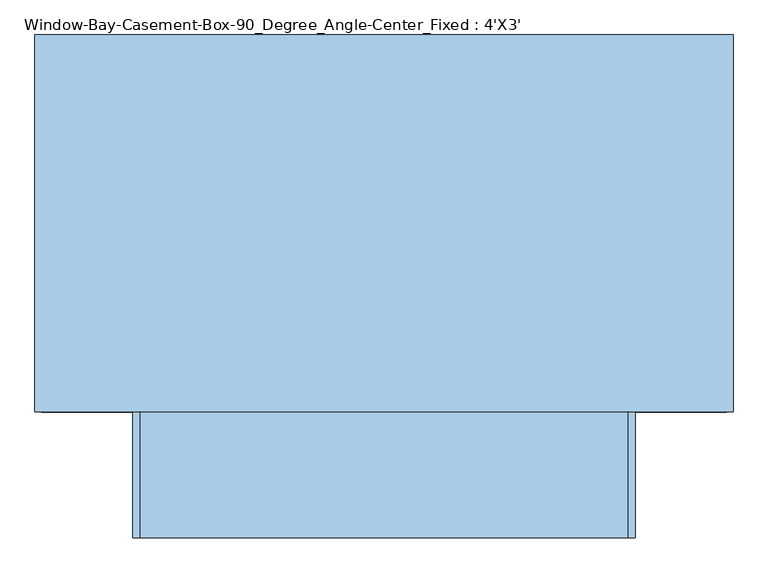
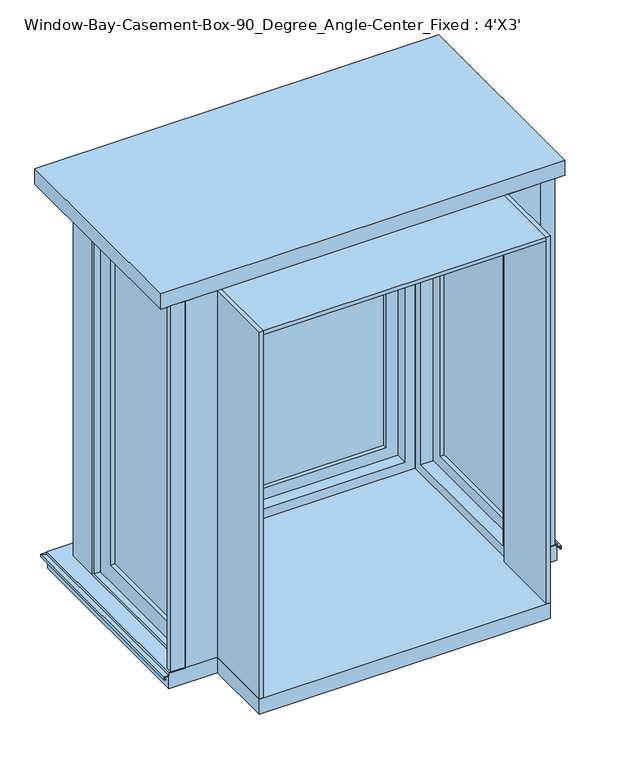
"""IFC4 building model written with IfcOpenShell, lengths in millimetres: window geometry, Window-Bay-Casement-Box-90_Degree_Angle-Center_Fixed : 4'X3'."""

from ifc_helpers import new_model, si_unit, frame, origin, place, context, project, spatial, polyline, outline, extrude, faceted_brep, source, transform, mapped, element, save


def window_bay_casement_box_90_degree_angle_center_fixed_4_x3_2dea7aab(model_context):
    return source(origin(), model_context, "Body", "SolidModel", [
        extrude(outline(polyline([(-558.8, 114.3), (-603.25, 114.3), (-603.25, 133.35), (-558.8, 133.35), (-558.8, 114.3)])), frame((0.0, 0.0, 663.1486341), z_axis=(0.0, 0.0, 1.0), x_axis=(1.0, 0.0, 0.0)), (0.0, 0.0, 1.0), 1216.4513659),
        extrude(outline(polyline([(603.25, 114.3), (558.8, 114.3), (558.8, 133.35), (603.25, 133.35), (603.25, 114.3)])), frame((0.0, 0.0, 663.1486341), z_axis=(0.0, 0.0, 1.0), x_axis=(1.0, 0.0, 0.0)), (0.0, 0.0, 1.0), 1216.4513659),
        faceted_brep([(-609.6, 114.3, 653.0697935), (-609.6, 114.3, 660.4), (-558.8, 114.3, 660.4), (-558.8, 114.3, 663.1486341), (-610.997, 114.3, 663.1486341), (-610.997, 114.3, 654.4483503), (-623.697, 114.3, 652.2089977), (-623.697, 114.3, 643.2668038), (-619.7346, 114.3, 643.2668038), (-619.7346, 114.3, 644.7270038), (-622.0968, 114.3, 644.7270038), (-622.0968, 114.3, 650.8662705), (609.6, 114.3, 653.0697935), (622.0968, 114.3, 650.8662705), (622.0968, 114.3, 644.7270038), (619.7346, 114.3, 644.7270038), (619.7346, 114.3, 643.2668038), (623.697, 114.3, 643.2668038), (623.697, 114.3, 652.2089977), (610.997, 114.3, 654.4483503), (610.997, 114.3, 663.1486341), (558.8, 114.3, 663.1486341), (558.8, 114.3, 660.4), (609.6, 114.3, 660.4), (-609.6, 774.7, 653.0697935), (-609.6, 774.7, 660.4), (609.6, 774.7, 660.4), (558.8, 723.9, 660.4), (-558.8, 723.9, 660.4), (-558.8, 723.9, 663.1486341), (558.8, 723.9, 663.1486341), (610.997, 776.097, 663.1486341), (-610.997, 776.097, 663.1486341), (-610.997, 776.097, 654.4483503), (-623.697, 788.797, 652.2089977), (-623.697, 788.797, 643.2668038), (623.697, 788.797, 643.2668038), (619.7346, 784.8346, 643.2668038), (-619.7346, 784.8346, 643.2668038), (-619.7346, 784.8346, 644.7270038), (619.7346, 784.8346, 644.7270038), (622.0968, 787.1968, 644.7270038), (-622.0968, 787.1968, 644.7270038), (-622.0968, 787.1968, 650.8662705), (609.6, 774.7, 653.0697935), (610.997, 776.097, 654.4483503), (623.697, 788.797, 652.2089977), (622.0968, 787.1968, 650.8662705)], [[[0, 1, 2, 3, 4, 5, 6, 7, 8, 9, 10, 11]], [[12, 13, 14, 15, 16, 17, 18, 19, 20, 21, 22, 23]], [[1, 0, 24, 25]], [[2, 1, 25, 26, 23, 22, 27, 28]], [[3, 2, 28, 29]], [[4, 3, 29, 30, 21, 20, 31, 32]], [[5, 4, 32, 33]], [[6, 5, 33, 34]], [[7, 6, 34, 35]], [[8, 7, 35, 36, 17, 16, 37, 38]], [[9, 8, 38, 39]], [[10, 9, 39, 40, 15, 14, 41, 42]], [[11, 10, 42, 43]], [[0, 11, 43, 24]], [[25, 24, 44, 26]], [[29, 28, 27, 30]], [[33, 32, 31, 45]], [[34, 33, 45, 46]], [[35, 34, 46, 36]], [[39, 38, 37, 40]], [[43, 42, 41, 47]], [[24, 43, 47, 44]], [[26, 44, 12, 23]], [[30, 27, 22, 21]], [[45, 31, 20, 19]], [[46, 45, 19, 18]], [[36, 46, 18, 17]], [[40, 37, 16, 15]], [[47, 41, 14, 13]], [[44, 47, 13, 12]]]),
        extrude(outline(polyline([(609.6, 774.7), (609.6, 114.3), (457.2, 114.3), (457.2, -114.3), (-457.2, -114.3), (-457.2, 114.3), (-609.6, 114.3), (-609.6, 774.7), (609.6, 774.7)])), frame((0.0, 0.0, 609.6), z_axis=(0.0, 0.0, 1.0), x_axis=(1.0, 0.0, 0.0)), (0.0, 0.0, 1.0), 50.8),
        extrude(outline(polyline([(635.0, 800.1), (635.0, 114.3), (-635.0, 114.3), (-635.0, 800.1), (635.0, 800.1)])), frame((0.0, 0.0, 1879.6), z_axis=(0.0, 0.0, 1.0), x_axis=(1.0, 0.0, 0.0)), (0.0, 0.0, 1.0), 50.8),
        extrude(outline(polyline([(-457.2, 723.9), (-457.2, 622.3), (-558.8, 622.3), (-558.8, 723.9), (-457.2, 723.9)])), frame((0.0, 0.0, 660.4), z_axis=(0.0, 0.0, 1.0), x_axis=(1.0, 0.0, 0.0)), (0.0, 0.0, 1.0), 1219.2),
        extrude(outline(polyline([(558.8, 723.9), (558.8, 622.3), (457.2, 622.3), (457.2, 723.9), (558.8, 723.9)])), frame((0.0, 0.0, 660.4), z_axis=(0.0, 0.0, 1.0), x_axis=(1.0, 0.0, 0.0)), (0.0, 0.0, 1.0), 1219.2),
        faceted_brep([(444.5, 660.4, 673.1), (444.5, 723.9, 673.1), (-444.5, 723.9, 673.1), (-444.5, 660.4, 673.1), (425.45, 622.3, 692.15), (425.45, 660.4, 692.15), (-425.45, 660.4, 692.15), (-425.45, 622.3, 692.15), (457.2, 723.9, 660.4), (457.2, 622.3, 660.4), (-457.2, 622.3, 660.4), (-457.2, 723.9, 660.4), (-444.5, 723.9, 1866.9), (-444.5, 660.4, 1866.9), (-425.45, 660.4, 1847.85), (-425.45, 622.3, 1847.85), (-457.2, 622.3, 1879.6), (-457.2, 723.9, 1879.6), (444.5, 723.9, 1866.9), (444.5, 660.4, 1866.9), (425.45, 660.4, 1847.85), (425.45, 622.3, 1847.85), (457.2, 622.3, 1879.6), (457.2, 723.9, 1879.6)], [[[0, 1, 2, 3]], [[4, 5, 6, 7]], [[8, 9, 10, 11]], [[3, 2, 12, 13]], [[7, 6, 14, 15]], [[11, 10, 16, 17]], [[13, 12, 18, 19]], [[15, 14, 20, 21]], [[17, 16, 22, 23]], [[11, 17, 23, 8], [1, 18, 12, 2]], [[19, 18, 1, 0]], [[3, 13, 19, 0], [5, 20, 14, 6]], [[21, 20, 5, 4]], [[9, 22, 16, 10], [7, 15, 21, 4]], [[23, 22, 9, 8]]]),
        extrude(outline(polyline([(1866.9, -444.5), (673.1, -444.5), (673.1, 444.5), (1866.9, 444.5), (1866.9, -444.5)]), holes=[polyline([(1809.75, 387.35), (730.25, 387.35), (730.25, -387.35), (1809.75, -387.35), (1809.75, 387.35)])]), frame((0.0, 660.4, 0.0), z_axis=(0.0, 1.0, 0.0), x_axis=(0.0, 0.0, 1.0)), (0.0, 0.0, 1.0), 44.45),
        faceted_brep([(-457.2, 146.05, 1847.85), (-495.3, 146.05, 1847.85), (-495.3, 590.55, 1847.85), (-457.2, 590.55, 1847.85), (-558.8, 114.3, 1879.6), (-457.2, 114.3, 1879.6), (-457.2, 622.3, 1879.6), (-558.8, 622.3, 1879.6), (-495.3, 127.0, 1866.9), (-558.8, 127.0, 1866.9), (-558.8, 609.6, 1866.9), (-495.3, 609.6, 1866.9), (-495.3, 590.55, 692.15), (-457.2, 590.55, 692.15), (-457.2, 622.3, 660.4), (-558.8, 622.3, 660.4), (-558.8, 609.6, 673.1), (-495.3, 609.6, 673.1), (-495.3, 146.05, 692.15), (-457.2, 146.05, 692.15), (-457.2, 114.3, 660.4), (-558.8, 114.3, 660.4), (-558.8, 127.0, 673.1), (-495.3, 127.0, 673.1)], [[[0, 1, 2, 3]], [[4, 5, 6, 7]], [[8, 9, 10, 11]], [[3, 2, 12, 13]], [[7, 6, 14, 15]], [[11, 10, 16, 17]], [[13, 12, 18, 19]], [[15, 14, 20, 21]], [[17, 16, 22, 23]], [[11, 17, 23, 8], [1, 18, 12, 2]], [[19, 18, 1, 0]], [[5, 20, 14, 6], [3, 13, 19, 0]], [[21, 20, 5, 4]], [[7, 15, 21, 4], [9, 22, 16, 10]], [[23, 22, 9, 8]]]),
        extrude(outline(polyline([(609.6, 1866.9), (609.6, 673.1), (127.0, 673.1), (127.0, 1866.9), (609.6, 1866.9)]), holes=[polyline([(184.15, 1809.75), (184.15, 730.25), (552.45, 730.25), (552.45, 1809.75), (184.15, 1809.75)])]), frame((-539.75, 0.0, 0.0), z_axis=(1.0, 0.0, 0.0), x_axis=(0.0, 1.0, 0.0)), (0.0, 0.0, 1.0), 44.45),
        faceted_brep([(495.3, 146.05, 1847.85), (457.2, 146.05, 1847.85), (457.2, 590.55, 1847.85), (495.3, 590.55, 1847.85), (558.8, 127.0, 1866.9), (495.3, 127.0, 1866.9), (495.3, 609.6, 1866.9), (558.8, 609.6, 1866.9), (457.2, 114.3, 1879.6), (558.8, 114.3, 1879.6), (558.8, 622.3, 1879.6), (457.2, 622.3, 1879.6), (457.2, 590.55, 692.15), (495.3, 590.55, 692.15), (495.3, 609.6, 673.1), (558.8, 609.6, 673.1), (558.8, 622.3, 660.4), (457.2, 622.3, 660.4), (457.2, 146.05, 692.15), (495.3, 146.05, 692.15), (495.3, 127.0, 673.1), (558.8, 127.0, 673.1), (558.8, 114.3, 660.4), (457.2, 114.3, 660.4)], [[[0, 1, 2, 3]], [[4, 5, 6, 7]], [[8, 9, 10, 11]], [[3, 2, 12, 13]], [[7, 6, 14, 15]], [[11, 10, 16, 17]], [[13, 12, 18, 19]], [[15, 14, 20, 21]], [[17, 16, 22, 23]], [[11, 17, 23, 8], [1, 18, 12, 2]], [[19, 18, 1, 0]], [[5, 20, 14, 6], [3, 13, 19, 0]], [[21, 20, 5, 4]], [[9, 22, 16, 10], [7, 15, 21, 4]], [[23, 22, 9, 8]]]),
        extrude(outline(polyline([(609.6, 1866.9), (609.6, 673.1), (127.0, 673.1), (127.0, 1866.9), (609.6, 1866.9)]), holes=[polyline([(184.15, 1809.75), (184.15, 730.25), (552.45, 730.25), (552.45, 1809.75), (184.15, 1809.75)])]), frame((495.3, 0.0, 0.0), z_axis=(1.0, 0.0, 0.0), x_axis=(0.0, 1.0, 0.0)), (0.0, 0.0, 1.0), 44.45),
        extrude(outline(polyline([(387.35, 692.15), (387.35, 685.8), (-387.35, 685.8), (-387.35, 692.15), (387.35, 692.15)])), frame((0.0, 0.0, 730.25), z_axis=(0.0, 0.0, 1.0), x_axis=(1.0, 0.0, 0.0)), (0.0, 0.0, 1.0), 1079.5),
        extrude(outline(polyline([(387.35, 679.45), (387.35, 673.1), (-387.35, 673.1), (-387.35, 679.45), (387.35, 679.45)])), frame((0.0, 0.0, 730.25), z_axis=(0.0, 0.0, 1.0), x_axis=(1.0, 0.0, 0.0)), (0.0, 0.0, 1.0), 1079.5),
        extrude(outline(polyline([(-520.7, 552.45), (-520.7, 184.15), (-527.05, 184.15), (-527.05, 552.45), (-520.7, 552.45)])), frame((0.0, 0.0, 730.25), z_axis=(0.0, 0.0, 1.0), x_axis=(1.0, 0.0, 0.0)), (0.0, 0.0, 1.0), 1079.5),
        extrude(outline(polyline([(-508.0, 552.45), (-508.0, 184.15), (-514.35, 184.15), (-514.35, 552.45), (-508.0, 552.45)])), frame((0.0, 0.0, 730.25), z_axis=(0.0, 0.0, 1.0), x_axis=(1.0, 0.0, 0.0)), (0.0, 0.0, 1.0), 1079.5),
        extrude(outline(polyline([(527.05, 552.45), (527.05, 184.15), (520.7, 184.15), (520.7, 552.45), (527.05, 552.45)])), frame((0.0, 0.0, 730.25), z_axis=(0.0, 0.0, 1.0), x_axis=(1.0, 0.0, 0.0)), (0.0, 0.0, 1.0), 1079.5),
        extrude(outline(polyline([(514.35, 552.45), (514.35, 184.15), (508.0, 184.15), (508.0, 552.45), (514.35, 552.45)])), frame((0.0, 0.0, 730.25), z_axis=(0.0, 0.0, 1.0), x_axis=(1.0, 0.0, 0.0)), (0.0, 0.0, 1.0), 1079.5),
        faceted_brep([(558.8, 127.0, 1866.9), (495.3, 127.0, 1866.9), (495.3, 609.6, 1866.9), (558.8, 609.6, 1866.9), (457.2, 114.3, 1879.6), (558.8, 114.3, 1879.6), (558.8, 622.3, 1879.6), (457.2, 622.3, 1879.6), (495.3, 146.05, 1847.85), (457.2, 146.05, 1847.85), (457.2, 590.55, 1847.85), (495.3, 590.55, 1847.85), (495.3, 609.6, 673.1), (558.8, 609.6, 673.1), (558.8, 622.3, 660.4), (457.2, 622.3, 660.4), (457.2, 590.55, 692.15), (495.3, 590.55, 692.15), (495.3, 127.0, 673.1), (558.8, 127.0, 673.1), (558.8, 114.3, 660.4), (457.2, 114.3, 660.4), (457.2, 146.05, 692.15), (495.3, 146.05, 692.15)], [[[0, 1, 2, 3]], [[4, 5, 6, 7]], [[8, 9, 10, 11]], [[3, 2, 12, 13]], [[7, 6, 14, 15]], [[11, 10, 16, 17]], [[13, 12, 18, 19]], [[15, 14, 20, 21]], [[17, 16, 22, 23]], [[1, 18, 12, 2], [11, 17, 23, 8]], [[19, 18, 1, 0]], [[5, 20, 14, 6], [3, 13, 19, 0]], [[21, 20, 5, 4]], [[7, 15, 21, 4], [9, 22, 16, 10]], [[23, 22, 9, 8]]]),
        extrude(outline(polyline([(-444.5, 114.3), (-444.5, -114.3), (-457.2, -114.3), (-457.2, 114.3), (-444.5, 114.3)])), frame((0.0, 0.0, 660.4), z_axis=(0.0, 0.0, 1.0), x_axis=(1.0, 0.0, 0.0)), (0.0, 0.0, 1.0), 1219.2),
        extrude(outline(polyline([(444.5, 114.3), (457.2, 114.3), (457.2, -114.3), (444.5, -114.3), (444.5, 114.3)])), frame((0.0, 0.0, 660.4), z_axis=(0.0, 0.0, 1.0), x_axis=(1.0, 0.0, 0.0)), (0.0, 0.0, 1.0), 1219.2),
        extrude(outline(polyline([(444.5, -114.3), (-444.5, -114.3), (-444.5, 622.3), (444.5, 622.3), (444.5, -114.3)])), frame((0.0, 0.0, 1866.9), z_axis=(0.0, 0.0, 1.0), x_axis=(1.0, 0.0, 0.0)), (0.0, 0.0, 1.0), 12.7),
    ])


if __name__ == "__main__":
    model = new_model("IFC4")
    model_context = context("Model", 3, world=origin())
    ifc_project = project(units=[si_unit("LENGTHUNIT", "METRE", prefix="MILLI")], contexts=[model_context])
    site = spatial("IfcSite", under=ifc_project)
    building = spatial("IfcBuilding", under=site)
    placement = place(None, origin())
    window_bay_casement_box_90_degree_angle_center_fixed_4_x3_shape = window_bay_casement_box_90_degree_angle_center_fixed_4_x3_2dea7aab(model_context)
    element("IfcWindow", 1, ObjectType="Window-Bay-Casement-Box-90_Degree_Angle-Center_Fixed : 4'X3'", at=placement, inside=building, context=model_context, shape_type="MappedRepresentation", body=[
        mapped(window_bay_casement_box_90_degree_angle_center_fixed_4_x3_shape, transform((0.0, 0.0, 0.0), x_axis=(1.0, 0.0, 0.0), y_axis=(0.0, 1.0, 0.0), z_axis=(0.0, 0.0, 1.0))),
    ])
    save(model, "model.ifc")

# Revit data of these elements
# Type "Window-Bay-Casement-Box-90_Degree_Angle-Center_Fixed : 4'X3'"
#   Type Mark = "19"
#   Fire Rating = "0.5h"
#   Assembly Code = "B2020100"
#   Analytic Construction = "1/8 in Pilkington single glazing"
#   Width = 3' - 0"
#   Wall Thickness [instance default] = 0' - 6"
#   Visual Light Transmittance = 0.9
#   Trim Width = 3' - 8"
#   Trim Height = 4' - 0"
#   Thermal Resistance (R) = 1.5394 (h·ft²·°F)/BTU
#   Solar Heat Gain Coefficient = 0.86
#   Rough Width = 3' - 0 1/2"
#   Rough Height = 4' - 0 1/2"
#   Height 1 = 4' - 2"
#   Height = 4' - 0"
#   Heat Transfer Coefficient (U) = 0.6496 BTU/(h·ft²·°F)
#   Depth = 2' - 0"
#   Default Sill Height = 2' - 0"
#   Side Muntin Visibility = yes
#   Center Muntin Visibility = yes
#   Interior Trim Visibility [instance default] = yes
#   Exterior Trim Visibility [instance default] = yes
#   Side Muntin Pattern = Muntin Pattern_2x2 : Muntin Pattern_2x2
#   Center Muntin Pattern = Muntin Pattern_2x2 : Muntin Pattern_2x2
#   Interior Trim Material = Wood - Stained
#   Exterior Trim Material = Clad - White
#   Exterior Trim = element 407684
#   Interior Trim = Trim-Window-Interior-Flat : Picture Frame
#   Interior Frame Material = Wood - Stained
#   Glass Panel Material = Glass
#   Exterior Frame Material = Clad - White
#   Wall Closure = (empty or 0)
# Element 1 (IfcWindow, "Window-Bay-Casement-Box-90_Degree_Angle-Center_Fixed : 4'X3'")
#   Wall Thickness = 0' - 9"
#   Materials on its faces: "Clad - White", "Wood - Stained", "Glass"
# Materials
#   "Wood - Stained": class "Wood", colour RGB 224 178 126, transparency 0, Cost = 0
#   "Clad - White": class "Wood", colour RGB 242 242 238, transparency 0, Cost = 0
#   "Glass": class "Glass", colour RGB 0 128 192, transparency 0.75, Description = "Soda Lime Glass", Cost = 0
